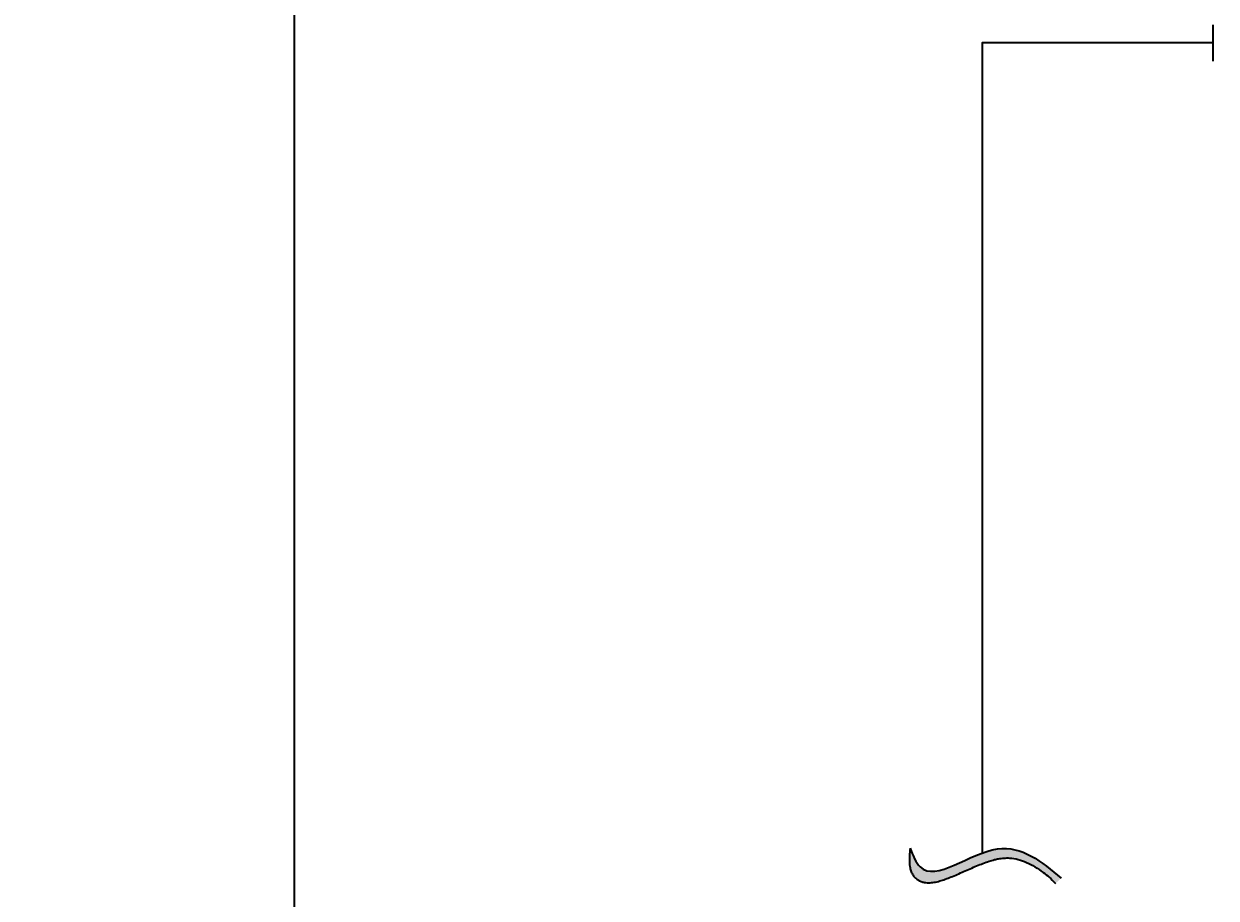
# Model space of a CAD drawing. Units: millimetres. Extents: x 353872 to 441597, y 126154 to 187356.
# Tile 17 of 28: x 391248 to 399262, y 161299 to 167178. Entities that reach past the tile are written whole.
import ezdxf

# ---------------------------------------------------------------- set-up
doc = ezdxf.new("R2010")
doc.units = ezdxf.units.MM
for name, color, linetype, lineweight in [('A-ANNO-DIMS', 2, 'Continuous', 18), ('P-PIPE', 3, 'Continuous', 35), ('P-SYMB-PATT', 8, 'Continuous', 13)]:
    doc.layers.add(name, color=color, linetype=linetype, lineweight=lineweight)
doc.styles.get("Standard").update_dxf_attribs({"font": 'arial.ttf'})
doc.dimstyles.get("Standard").update_dxf_attribs({"dimtxt": 0.18, "dimasz": 0.18, "dimexe": 0.18, "dimexo": 0.0625, "dimgap": 0.09, "dimtad": 0, "dimtih": 1, "dimtoh": 1, "dimdec": 4, "dimzin": 0, "dimdsep": 46, "dimtxsty": 'Standard', "dimcen": 0.09, "dimadec": 0, "dimazin": 0, "dimtfac": 1, "dimtdec": 4, "dimtofl": 0, "dimtmove": 0, "dimatfit": 3, "dimfxl": 1, "dimtolj": 1, "dimtzin": 0, "dimarcsym": 0})

# ---------------------------------------------------------------- blocks, each defined once
blk = doc.blocks.new('*D34')
at = {"layer": 'A-ANNO-DIMS', "color": 0, "lineweight": -2, "transparency": 16777216}
for p, q in [((399457.1, 167930), (356736.4, 167930)), ((356736.5, 167929.8), (356736.5, 163994.3)), ((356736.5, 160058.4), (356736.5, 163993.9)), ((399457.1, 160058.2), (356736.4, 160058.2))]:
    blk.add_line(p, q, dxfattribs=at)
at = {"layer": 'A-ANNO-DIMS', "color": 0, "transparency": 16777216}
for points in [[(356736.5, 167929.8), (356736.6, 167929.8), (356736.5, 167930)], [(356736.5, 160058.4), (356736.6, 160058.4), (356736.5, 160058.2)]]:
    blk.add_solid(points, dxfattribs=at)
at = {"layer": 'Defpoints', "color": 0, "transparency": 16777216}
for p in [(399457.2, 167930), (356736.5, 160058.2), (399457.2, 160058.2)]:
    blk.add_point(p, dxfattribs=at)
at = {"layer": 'A-ANNO-DIMS', "color": 0, "transparency": 16777216, "insert": (356736.5, 163994.1), "char_height": 0.18, "attachment_point": 5}
blk.add_mtext('\\A1;7872', dxfattribs=at)

msp = doc.modelspace()

# ---------------------------------------------------------------- hatches: boundary and pattern name
at = {"layer": 'P-SYMB-PATT'}
h = msp.add_hatch(color=256, dxfattribs=at)
h.dxf.hatch_style = 1
edge = h.paths.add_edge_path()
edge.add_spline(control_points=[(397205.05, 161635.73), (397204.61, 161630.78), (397204.16, 161625.76), (397202.84, 161610.6), (397202.01, 161600.34), (397200.63, 161578.85), (397200.12, 161567.62), (397199.95, 161545.12), (397200.28, 161533.87), (397202.07, 161516.2), (397202.95, 161509.94), (397205.13, 161498.92), (397206.25, 161494.21), (397209.06, 161484.65), (397210.73, 161479.9), (397215.91, 161467.48), (397219.95, 161459.9), (397229.78, 161445.61), (397235.58, 161438.93), (397248.52, 161427.16), (397255.64, 161422.09), (397270.38, 161413.86), (397277.98, 161410.69), (397293.04, 161405.96), (397300.51, 161404.38), (397315.1, 161402.39), (397322.23, 161401.97), (397342.23, 161401.93), (397354.76, 161403.27), (397379.55, 161407.54), (397391.81, 161410.5), (397416.54, 161417.55), (397428.98, 161421.66), (397454.23, 161430.73), (397467.03, 161435.69), (397507.59, 161452.16), (397536.01, 161464.73), (397593.65, 161490.26), (397622.85, 161503.21), (397680.46, 161527.08), (397708.87, 161537.99), (397748.65, 161550.84), (397761.14, 161554.49), (397781.84, 161559.73), (397790.28, 161561.61), (397805.08, 161564.41), (397811.57, 161565.44), (397824.38, 161567.1), (397830.66, 161567.71), (397849.19, 161568.98), (397861.12, 161569.06), (397893.15, 161567.36), (397912.63, 161564.19), (397950.84, 161554.2), (397969.58, 161547.37), (398006.91, 161530.44), (398025.48, 161520.34), (398062.71, 161497.47), (398081.36, 161484.7), (398126.14, 161452.04), (398152.38, 161431.3), (398181.22, 161397.19)], knot_values=[0, 0, 0, 0, 1.456577, 1.456577, 4.3697309, 4.3697309, 7.5343006, 7.5343006, 10.6988703, 10.6988703, 12.406712, 12.406712, 13.6390126, 13.6390126, 14.8713131, 14.8713131, 16.9006125, 16.9006125, 18.9299119, 18.9299119, 20.9592113, 20.9592113, 22.9885107, 22.9885107, 25.01781, 25.01781, 27.0471094, 27.0471094, 30.8253225, 30.8253225, 34.6035357, 34.6035357, 38.3817488, 38.3817488, 42.1599619, 42.1599619, 50.1898356, 50.1898356, 58.2197092, 58.2197092, 66.2495828, 66.2495828, 70.07412, 70.07412, 72.8401263, 72.8401263, 75.120346, 75.120346, 77.4005658, 77.4005658, 81.9610053, 81.9610053, 89.9551657, 89.9551657, 97.9493262, 97.9493262, 105.9434867, 105.9434867, 113.9376472, 113.9376472, 125.0020106, 125.0020106, 125.0020106, 125.0020106], degree=3, periodic=0)
edge.add_line((398181.22, 161397.19), (398220.74, 161433.13))
edge.add_spline(control_points=[(398220.74, 161433.13), (398088.6, 161543.3), (397930.06, 161675.49), (397724.17, 161614.98), (397689.5, 161602.16)], knot_values=[65.2965705, 65.2965705, 65.2965705, 65.2965705, 118.2135452, 128.7852065, 128.7852065, 128.7852065, 128.7852065], degree=3, periodic=0)
edge.add_spline(control_points=[(397689.5, 161602.16), (397527.98, 161542.5), (397302.36, 161384.72), (397224.26, 161586.19), (397205.05, 161635.73)], knot_values=[0, 0, 0, 0, 49.2381661, 65.2965705, 65.2965705, 65.2965705, 65.2965705], degree=3, periodic=0)

# ---------------------------------------------------------------- linework, layer by layer
at = {"layer": 'P-PIPE'}
msp.add_line((399242.2, 166926.77), (399242.2, 167171.53), dxfattribs=at)
for points in [[(393066.71, 149319.73), (393066.71, 175399.89), (426420.76, 175399.89)], [(399242.2, 167049.15), (397689.5, 167049.15), (397689.5, 161602.16)]]:
    msp.add_lwpolyline(points, dxfattribs=at)
for points, knots in [([(397205.05, 161635.73), (397204.61, 161630.78), (397204.16, 161625.76), (397202.84, 161610.6), (397202.01, 161600.34), (397200.63, 161578.85), (397200.12, 161567.62), (397199.95, 161545.12), (397200.28, 161533.87), (397202.07, 161516.2), (397202.95, 161509.94), (397205.13, 161498.92), (397206.25, 161494.21), (397209.06, 161484.65), (397210.73, 161479.9), (397215.91, 161467.48), (397219.95, 161459.9), (397229.78, 161445.61), (397235.58, 161438.93), (397248.52, 161427.16), (397255.64, 161422.09), (397270.38, 161413.86), (397277.98, 161410.69), (397293.04, 161405.96), (397300.51, 161404.38), (397315.1, 161402.39), (397322.23, 161401.97), (397342.23, 161401.93), (397354.76, 161403.27), (397379.55, 161407.54), (397391.81, 161410.5), (397416.54, 161417.55), (397428.98, 161421.66), (397454.23, 161430.73), (397467.03, 161435.69), (397507.59, 161452.16), (397536.01, 161464.73), (397593.65, 161490.26), (397622.85, 161503.21), (397680.46, 161527.08), (397708.87, 161537.99), (397748.65, 161550.84), (397761.14, 161554.49), (397781.84, 161559.73), (397790.28, 161561.61), (397805.08, 161564.41), (397811.57, 161565.44), (397824.38, 161567.1), (397830.66, 161567.71), (397849.19, 161568.98), (397861.12, 161569.06), (397893.15, 161567.36), (397912.63, 161564.19), (397950.84, 161554.2), (397969.58, 161547.37), (398006.91, 161530.44), (398025.48, 161520.34), (398062.71, 161497.47), (398081.36, 161484.7), (398126.14, 161452.04), (398152.38, 161431.3), (398181.22, 161397.19)], [0, 0, 0, 0, 1.456577, 1.456577, 4.3697309, 4.3697309, 7.5343006, 7.5343006, 10.6988703, 10.6988703, 12.406712, 12.406712, 13.6390126, 13.6390126, 14.8713131, 14.8713131, 16.9006125, 16.9006125, 18.9299119, 18.9299119, 20.9592113, 20.9592113, 22.9885107, 22.9885107, 25.01781, 25.01781, 27.0471094, 27.0471094, 30.8253225, 30.8253225, 34.6035357, 34.6035357, 38.3817488, 38.3817488, 42.1599619, 42.1599619, 50.1898356, 50.1898356, 58.2197092, 58.2197092, 66.2495828, 66.2495828, 70.07412, 70.07412, 72.8401263, 72.8401263, 75.120346, 75.120346, 77.4005658, 77.4005658, 81.9610053, 81.9610053, 89.9551657, 89.9551657, 97.9493262, 97.9493262, 105.9434867, 105.9434867, 113.9376472, 113.9376472, 125.0020106, 125.0020106, 125.0020106, 125.0020106]), ([(397205.05, 161635.73), (397224.26, 161586.19), (397315, 161352.1), (397807.1, 161778.01), (398088.6, 161543.3), (398220.74, 161433.13)], [0, 0, 0, 0, 143.2990836, 677.0191991, 1149.2301239, 1149.2301239, 1149.2301239, 1149.2301239])]:
    msp.add_open_spline(points, degree=3, knots=knots, dxfattribs=at)

# ---------------------------------------------------------------- dimensions: what is measured, and where the dimension line sits
at = {"layer": 'A-ANNO-DIMS'}
dim = msp.add_linear_dim(base=(356736.55, 160058.19), p1=(399457.15, 167929.97), p2=(399457.15, 160058.19), angle=90, dimstyle='Standard', override={"dimdec": 0, "dimlfac": 1, "dimrnd": 0, "dimzin": 0, "dimdsep": 46, "dimlunit": 2}, dxfattribs=at)
dim.commit()
dim.dimension.update_dxf_attribs({"geometry": '*D34', "text_midpoint": (356736.55, 163994.08)})

doc.saveas('drawing.dxf')
